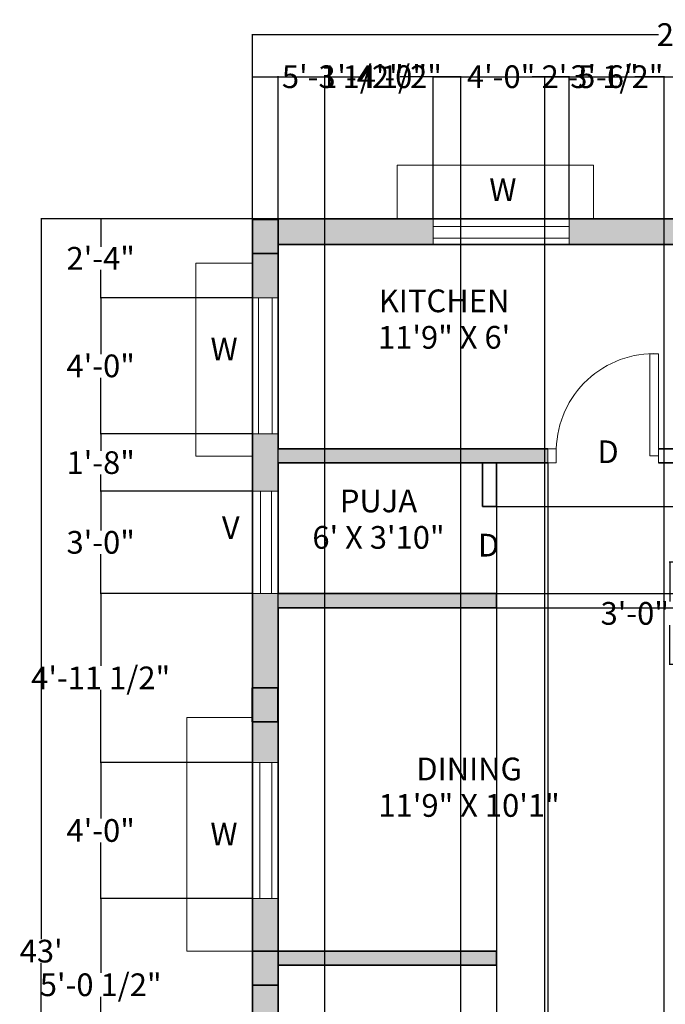
# Model space of a CAD drawing. Units: inches. Extents: x 374 to 1054, y -870 to -188.
# Tile 2 of 3: x 374 to 601, y -535 to -188. Entities that reach past the tile are written whole.
import ezdxf
from ezdxf.enums import TextEntityAlignment as Align

# ---------------------------------------------------------------- set-up
doc = ezdxf.new("R2010")
doc.units = ezdxf.units.IN
doc.header["$MEASUREMENT"] = 0
for name, color, linetype, lineweight, true_color in [('A-ANNO-DIMS', 244, 'Continuous', 18, 0x991b1e), ('A-AREA-IDEN', 116, 'Continuous', 18, 0x136734), ('A-WALL-PATT', 116, 'Continuous', 13, 0x136734)]:
    doc.layers.add(name, color=color, linetype=linetype, lineweight=lineweight, true_color=true_color)
for name, color, linetype, lineweight in [('A-ANNO-TEXT', 7, 'Continuous', 18), ('A-COLS', 1, 'Continuous', 35), ('A-DOOR', 4, 'Continuous', 18), ('A-FLOR-CASE-PATT', 8, 'Continuous', 13), ('A-GLAZ', 4, 'Continuous', 18), ('A-GLAZ-PROJ', 4, 'Continuous', 13), ('A-WALL', 7, 'Continuous', 35)]:
    doc.layers.add(name, color=color, linetype=linetype, lineweight=lineweight)
doc.styles.get("Standard").update_dxf_attribs({"font": 'arial.ttf'})
doc.dimstyles.get("Standard").update_dxf_attribs({"dimtxt": 8, "dimasz": 0.18, "dimexe": 0.18, "dimexo": 0.0625, "dimgap": 0.09, "dimtad": 0, "dimtih": 1, "dimtoh": 1, "dimzin": 0, "dimdsep": 46, "dimlunit": 3, "dimtxsty": 'Standard', "dimcen": 0.09, "dimadec": 0, "dimazin": 0, "dimtfac": 1, "dimtofl": 0, "dimtmove": 0, "dimatfit": 3, "dimfxl": 1, "dimtolj": 1, "dimtzin": 0, "dimarcsym": 0})

# ---------------------------------------------------------------- blocks, each defined once
blk = doc.blocks.new('*D1')
at = {"layer": 'A-ANNO-DIMS', "color": 0, "lineweight": -2, "transparency": 16777216}
for p, q in [((455.9, -257.88), (455.9, -192.83)), ((456.08, -193.01), (598.96, -193.01)), ((755.72, -193.01), (612.85, -193.01)), ((755.9, -257.88), (755.9, -192.83))]:
    blk.add_line(p, q, dxfattribs=at)
at = {"layer": 'A-ANNO-DIMS', "color": 0, "transparency": 16777216}
for points in [[(456.08, -192.98), (456.08, -193.04), (455.9, -193.01)], [(755.72, -192.98), (755.72, -193.04), (755.9, -193.01)]]:
    blk.add_solid(points, dxfattribs=at)
at = {"layer": 'Defpoints', "color": 0, "transparency": 16777216}
for p in [(755.9, -193.01), (455.9, -257.94), (755.9, -257.94)]:
    blk.add_point(p, dxfattribs=at)
at = {"layer": 'A-ANNO-DIMS', "color": 0, "transparency": 16777216, "insert": (605.9, -193.01), "char_height": 8, "attachment_point": 5}
blk.add_mtext("\\A1;25'", dxfattribs=at)
blk = doc.blocks.new('*D2')
at = {"layer": 'A-ANNO-DIMS', "color": 0, "lineweight": -2, "transparency": 16777216}
for p, q in [((455.84, -257.94), (381.2, -257.94)), ((381.38, -258.12), (381.38, -511.76)), ((381.38, -773.76), (381.38, -520.12)), ((455.84, -773.94), (381.2, -773.94))]:
    blk.add_line(p, q, dxfattribs=at)
at = {"layer": 'A-ANNO-DIMS', "color": 0, "transparency": 16777216}
for points in [[(381.35, -258.12), (381.41, -258.12), (381.38, -257.94)], [(381.35, -773.76), (381.41, -773.76), (381.38, -773.94)]]:
    blk.add_solid(points, dxfattribs=at)
at = {"layer": 'Defpoints', "color": 0, "transparency": 16777216}
for p in [(381.38, -257.94), (455.9, -257.94), (455.9, -773.94)]:
    blk.add_point(p, dxfattribs=at)
at = {"layer": 'A-ANNO-DIMS', "color": 0, "transparency": 16777216, "insert": (381.38, -515.94), "char_height": 8, "attachment_point": 5}
blk.add_mtext("\\A1;43'", dxfattribs=at)
blk = doc.blocks.new('COL-12X9')
h = blk.add_hatch(color=256)
h.dxf.hatch_style = 1
h.paths.add_polyline_path([(6, 4.5), (-6, 4.5), (-6, -4.5), (6, -4.5)])
blk.add_lwpolyline([(-6, 4.5), (6, 4.5), (6, -4.5), (-6, -4.5)], close=True)
blk = doc.blocks.new('DOOR-SWING-36')
blk.add_lwpolyline([(0, 0), (-3, 0), (-3, 36), (0, 36)], close=True)
blk.add_arc((-1.5, 1.52), 34.51, 87.5091, 178.3707)
blk = doc.blocks.new('*D9')
at = {"layer": 'A-ANNO-DIMS', "color": 0, "lineweight": -2, "transparency": 16777216}
for p, q in [((608.34, -378.94), (602.76, -378.94)), ((602.94, -379.12), (602.94, -392.76)), ((602.94, -414.76), (602.94, -401.12)), ((608.34, -414.94), (602.76, -414.94))]:
    blk.add_line(p, q, dxfattribs=at)
at = {"layer": 'A-ANNO-DIMS', "color": 0, "transparency": 16777216}
for points in [[(602.91, -379.12), (602.97, -379.12), (602.94, -378.94)], [(602.91, -414.76), (602.97, -414.76), (602.94, -414.94)]]:
    blk.add_solid(points, dxfattribs=at)
at = {"layer": 'Defpoints', "color": 0, "transparency": 16777216}
for p in [(608.4, -378.94), (602.94, -414.94), (608.4, -414.94)]:
    blk.add_point(p, dxfattribs=at)
at = {"layer": 'A-ANNO-DIMS', "color": 0, "transparency": 16777216, "insert": (602.94, -396.94), "char_height": 8, "attachment_point": 5}
blk.add_mtext('\\A1;3\'-0" TYP.', dxfattribs=at)
blk = doc.blocks.new('*D12')
at = {"layer": 'A-ANNO-DIMS', "color": 0, "lineweight": -2, "transparency": 16777216}
for p, q in [((455.9, -257.88), (455.9, -207.66)), ((456.08, -207.84), (467.65, -207.84)), ((519.3, -207.84), (507.74, -207.84)), ((519.48, -257.88), (519.48, -207.66))]:
    blk.add_line(p, q, dxfattribs=at)
at = {"layer": 'A-ANNO-DIMS', "color": 0, "transparency": 16777216}
for points in [[(456.08, -207.81), (456.08, -207.87), (455.9, -207.84)], [(519.3, -207.81), (519.3, -207.87), (519.48, -207.84)]]:
    blk.add_solid(points, dxfattribs=at)
at = {"layer": 'Defpoints', "color": 0, "transparency": 16777216}
for p in [(519.48, -207.84), (455.9, -257.94), (519.48, -257.94)]:
    blk.add_point(p, dxfattribs=at)
at = {"layer": 'A-ANNO-DIMS', "color": 0, "transparency": 16777216, "insert": (487.69, -207.84), "char_height": 8, "attachment_point": 5}
blk.add_mtext('\\A1;5\'-3 1/2"', dxfattribs=at)
blk = doc.blocks.new('*D13')
at = {"layer": 'A-ANNO-DIMS', "color": 0, "lineweight": -2, "transparency": 16777216}
for p, q in [((519.48, -257.88), (519.48, -207.66)), ((519.66, -207.84), (532.6, -207.84)), ((567.3, -207.84), (554.37, -207.84)), ((567.48, -257.88), (567.48, -207.66))]:
    blk.add_line(p, q, dxfattribs=at)
at = {"layer": 'A-ANNO-DIMS', "color": 0, "transparency": 16777216}
for points in [[(519.66, -207.81), (519.66, -207.87), (519.48, -207.84)], [(567.3, -207.81), (567.3, -207.87), (567.48, -207.84)]]:
    blk.add_solid(points, dxfattribs=at)
at = {"layer": 'Defpoints', "color": 0, "transparency": 16777216}
for p in [(567.48, -207.84), (519.48, -257.94), (567.48, -257.94)]:
    blk.add_point(p, dxfattribs=at)
at = {"layer": 'A-ANNO-DIMS', "color": 0, "transparency": 16777216, "insert": (543.48, -207.84), "char_height": 8, "attachment_point": 5}
blk.add_mtext('\\A1;4\'-0"', dxfattribs=at)
blk = doc.blocks.new('*D14')
at = {"layer": 'A-ANNO-DIMS', "color": 0, "lineweight": -2, "transparency": 16777216}
for p, q in [((567.48, -257.88), (567.48, -207.66)), ((567.66, -207.84), (606.87, -207.84)), ((667.53, -207.84), (628.32, -207.84)), ((667.71, -257.88), (667.71, -207.66))]:
    blk.add_line(p, q, dxfattribs=at)
at = {"layer": 'A-ANNO-DIMS', "color": 0, "transparency": 16777216}
for points in [[(567.66, -207.81), (567.66, -207.87), (567.48, -207.84)], [(667.53, -207.81), (667.53, -207.87), (667.71, -207.84)]]:
    blk.add_solid(points, dxfattribs=at)
at = {"layer": 'Defpoints', "color": 0, "transparency": 16777216}
for p in [(667.71, -207.84), (567.48, -257.94), (667.71, -257.94)]:
    blk.add_point(p, dxfattribs=at)
at = {"layer": 'A-ANNO-DIMS', "color": 0, "transparency": 16777216, "insert": (617.6, -207.84), "char_height": 8, "attachment_point": 5}
blk.add_mtext('\\A1;8\'-4"', dxfattribs=at)
blk = doc.blocks.new('*D16')
at = {"layer": 'A-ANNO-DIMS', "color": 0, "lineweight": -2, "transparency": 16777216}
for p, q in [((455.84, -257.94), (402.18, -257.94)), ((402.36, -258.12), (402.36, -267.73)), ((402.36, -285.55), (402.36, -275.94)), ((455.84, -285.73), (402.18, -285.73))]:
    blk.add_line(p, q, dxfattribs=at)
at = {"layer": 'A-ANNO-DIMS', "color": 0, "transparency": 16777216}
for points in [[(402.33, -258.12), (402.39, -258.12), (402.36, -257.94)], [(402.33, -285.55), (402.39, -285.55), (402.36, -285.73)]]:
    blk.add_solid(points, dxfattribs=at)
at = {"layer": 'Defpoints', "color": 0, "transparency": 16777216}
for p in [(455.9, -257.94), (402.36, -285.73), (455.9, -285.73)]:
    blk.add_point(p, dxfattribs=at)
at = {"layer": 'A-ANNO-DIMS', "color": 0, "transparency": 16777216, "insert": (402.36, -271.83), "char_height": 8, "attachment_point": 5}
blk.add_mtext('\\A1;2\'-4"', dxfattribs=at)
blk = doc.blocks.new('*D17')
at = {"layer": 'A-ANNO-DIMS', "color": 0, "lineweight": -2, "transparency": 16777216}
for p, q in [((455.84, -285.73), (402.18, -285.73)), ((402.36, -285.91), (402.36, -305.56)), ((402.36, -333.55), (402.36, -313.9)), ((455.84, -333.73), (402.18, -333.73))]:
    blk.add_line(p, q, dxfattribs=at)
at = {"layer": 'A-ANNO-DIMS', "color": 0, "transparency": 16777216}
for points in [[(402.33, -285.91), (402.39, -285.91), (402.36, -285.73)], [(402.33, -333.55), (402.39, -333.55), (402.36, -333.73)]]:
    blk.add_solid(points, dxfattribs=at)
at = {"layer": 'Defpoints', "color": 0, "transparency": 16777216}
for p in [(455.9, -285.73), (402.36, -333.73), (455.9, -333.73)]:
    blk.add_point(p, dxfattribs=at)
at = {"layer": 'A-ANNO-DIMS', "color": 0, "transparency": 16777216, "insert": (402.36, -309.73), "char_height": 8, "attachment_point": 5}
blk.add_mtext('\\A1;4\'-0"', dxfattribs=at)
blk = doc.blocks.new('*D18')
at = {"layer": 'A-ANNO-DIMS', "color": 0, "lineweight": -2, "transparency": 16777216}
for p, q in [((455.84, -333.73), (402.18, -333.73)), ((402.36, -333.91), (402.36, -339.64)), ((402.36, -353.73), (402.36, -347.99)), ((455.84, -353.91), (402.18, -353.91))]:
    blk.add_line(p, q, dxfattribs=at)
at = {"layer": 'A-ANNO-DIMS', "color": 0, "transparency": 16777216}
for points in [[(402.33, -333.91), (402.39, -333.91), (402.36, -333.73)], [(402.33, -353.73), (402.39, -353.73), (402.36, -353.91)]]:
    blk.add_solid(points, dxfattribs=at)
at = {"layer": 'Defpoints', "color": 0, "transparency": 16777216}
for p in [(455.9, -333.73), (402.36, -353.91), (455.9, -353.91)]:
    blk.add_point(p, dxfattribs=at)
at = {"layer": 'A-ANNO-DIMS', "color": 0, "transparency": 16777216, "insert": (402.36, -343.82), "char_height": 8, "attachment_point": 5}
blk.add_mtext('\\A1;1\'-8"', dxfattribs=at)
blk = doc.blocks.new('*D19')
at = {"layer": 'A-ANNO-DIMS', "color": 0, "lineweight": -2, "transparency": 16777216}
for p, q in [((455.84, -353.91), (402.18, -353.91)), ((402.36, -354.09), (402.36, -367.73)), ((402.36, -389.73), (402.36, -376.09)), ((455.84, -389.91), (402.18, -389.91))]:
    blk.add_line(p, q, dxfattribs=at)
at = {"layer": 'A-ANNO-DIMS', "color": 0, "transparency": 16777216}
for points in [[(402.33, -354.09), (402.39, -354.09), (402.36, -353.91)], [(402.33, -389.73), (402.39, -389.73), (402.36, -389.91)]]:
    blk.add_solid(points, dxfattribs=at)
at = {"layer": 'Defpoints', "color": 0, "transparency": 16777216}
for p in [(455.9, -353.91), (402.36, -389.91), (455.9, -389.91)]:
    blk.add_point(p, dxfattribs=at)
at = {"layer": 'A-ANNO-DIMS', "color": 0, "transparency": 16777216, "insert": (402.36, -371.91), "char_height": 8, "attachment_point": 5}
blk.add_mtext('\\A1;3\'-0"', dxfattribs=at)
blk = doc.blocks.new('*D20')
at = {"layer": 'A-ANNO-DIMS', "color": 0, "lineweight": -2, "transparency": 16777216}
for p, q in [((455.84, -389.91), (402.18, -389.91)), ((402.36, -390.09), (402.36, -415.44)), ((402.36, -449.25), (402.36, -423.9)), ((455.84, -449.43), (402.18, -449.43))]:
    blk.add_line(p, q, dxfattribs=at)
at = {"layer": 'A-ANNO-DIMS', "color": 0, "transparency": 16777216}
for points in [[(402.33, -390.09), (402.39, -390.09), (402.36, -389.91)], [(402.33, -449.25), (402.39, -449.25), (402.36, -449.43)]]:
    blk.add_solid(points, dxfattribs=at)
at = {"layer": 'Defpoints', "color": 0, "transparency": 16777216}
for p in [(455.9, -389.91), (402.36, -449.43), (455.9, -449.43)]:
    blk.add_point(p, dxfattribs=at)
at = {"layer": 'A-ANNO-DIMS', "color": 0, "transparency": 16777216, "insert": (402.36, -419.67), "char_height": 8, "attachment_point": 5}
blk.add_mtext('\\A1;4\'-11 1/2"', dxfattribs=at)
blk = doc.blocks.new('*D21')
at = {"layer": 'A-ANNO-DIMS', "color": 0, "lineweight": -2, "transparency": 16777216}
for p, q in [((455.84, -449.43), (402.18, -449.43)), ((402.36, -449.61), (402.36, -469.26)), ((402.36, -497.25), (402.36, -477.61)), ((455.84, -497.43), (402.18, -497.43))]:
    blk.add_line(p, q, dxfattribs=at)
at = {"layer": 'A-ANNO-DIMS', "color": 0, "transparency": 16777216}
for points in [[(402.33, -449.61), (402.39, -449.61), (402.36, -449.43)], [(402.33, -497.25), (402.39, -497.25), (402.36, -497.43)]]:
    blk.add_solid(points, dxfattribs=at)
at = {"layer": 'Defpoints', "color": 0, "transparency": 16777216}
for p in [(455.9, -449.43), (402.36, -497.43), (455.9, -497.43)]:
    blk.add_point(p, dxfattribs=at)
at = {"layer": 'A-ANNO-DIMS', "color": 0, "transparency": 16777216, "insert": (402.36, -473.43), "char_height": 8, "attachment_point": 5}
blk.add_mtext('\\A1;4\'-0"', dxfattribs=at)
blk = doc.blocks.new('*D22')
at = {"layer": 'A-ANNO-DIMS', "color": 0, "lineweight": -2, "transparency": 16777216}
for p, q in [((455.84, -497.43), (402.18, -497.43)), ((402.36, -497.61), (402.36, -523.56)), ((402.36, -557.96), (402.36, -532.01)), ((455.84, -558.14), (402.18, -558.14))]:
    blk.add_line(p, q, dxfattribs=at)
at = {"layer": 'A-ANNO-DIMS', "color": 0, "transparency": 16777216}
for points in [[(402.33, -497.61), (402.39, -497.61), (402.36, -497.43)], [(402.33, -557.96), (402.39, -557.96), (402.36, -558.14)]]:
    blk.add_solid(points, dxfattribs=at)
at = {"layer": 'Defpoints', "color": 0, "transparency": 16777216}
for p in [(455.9, -497.43), (402.36, -558.14), (455.9, -558.14)]:
    blk.add_point(p, dxfattribs=at)
at = {"layer": 'A-ANNO-DIMS', "color": 0, "transparency": 16777216, "insert": (402.36, -527.79), "char_height": 8, "attachment_point": 5}
blk.add_mtext('\\A1;5\'-0 1/2"', dxfattribs=at)
blk = doc.blocks.new('*D25')
at = {"layer": 'A-ANNO-DIMS', "color": 0, "lineweight": -2, "transparency": 16777216}
for p, q in [((541.93, -389.94), (810.73, -389.94)), ((810.55, -390.12), (810.55, -394.76)), ((541.92, -394.94), (810.73, -394.94)), ((810.55, -395.12), (810.37, -395.12)), ((810.55, -394.94), (810.55, -395.12))]:
    blk.add_line(p, q, dxfattribs=at)
at = {"layer": 'A-ANNO-DIMS', "color": 0, "transparency": 16777216}
for points in [[(810.52, -390.12), (810.58, -390.12), (810.55, -389.94)], [(810.52, -394.76), (810.58, -394.76), (810.55, -394.94)]]:
    blk.add_solid(points, dxfattribs=at)
at = {"layer": 'Defpoints', "color": 0, "transparency": 16777216}
for p in [(541.86, -389.94), (541.86, -394.94), (810.55, -394.94)]:
    blk.add_point(p, dxfattribs=at)
at = {"layer": 'A-ANNO-DIMS', "color": 0, "transparency": 16777216, "insert": (799.65, -395.12), "char_height": 8, "attachment_point": 5}
blk.add_mtext('\\A1;0\'-5"', dxfattribs=at)
blk = doc.blocks.new('*D39')
at = {"layer": 'A-ANNO-DIMS', "color": 0, "lineweight": -2, "transparency": 16777216}
for p, q in [((464.9, -680.88), (464.9, -207.66)), ((465.08, -207.84), (481.13, -207.84)), ((481.31, -680.88), (481.31, -207.66)), ((481.31, -207.84), (481.49, -207.84))]:
    blk.add_line(p, q, dxfattribs=at)
at = {"layer": 'A-ANNO-DIMS', "color": 0, "transparency": 16777216}
for points in [[(465.08, -207.81), (465.08, -207.87), (464.9, -207.84)], [(481.13, -207.81), (481.13, -207.87), (481.31, -207.84)]]:
    blk.add_solid(points, dxfattribs=at)
at = {"layer": 'Defpoints', "color": 0, "transparency": 16777216}
for p in [(481.31, -207.84), (464.9, -680.94), (481.31, -680.94)]:
    blk.add_point(p, dxfattribs=at)
at = {"layer": 'A-ANNO-DIMS', "color": 0, "transparency": 16777216, "insert": (501.16, -207.84), "char_height": 8, "attachment_point": 5}
blk.add_mtext('\\A1;1\'-4 1/2"', dxfattribs=at)
blk = doc.blocks.new('*D40')
at = {"layer": 'A-ANNO-DIMS', "color": 0, "lineweight": -2, "transparency": 16777216}
for p, q in [((481.31, -680.88), (481.31, -207.66)), ((481.49, -207.84), (494.43, -207.84)), ((529.13, -207.84), (516.2, -207.84)), ((529.31, -680.88), (529.31, -207.66))]:
    blk.add_line(p, q, dxfattribs=at)
at = {"layer": 'A-ANNO-DIMS', "color": 0, "transparency": 16777216}
for points in [[(481.49, -207.81), (481.49, -207.87), (481.31, -207.84)], [(529.13, -207.81), (529.13, -207.87), (529.31, -207.84)]]:
    blk.add_solid(points, dxfattribs=at)
at = {"layer": 'Defpoints', "color": 0, "transparency": 16777216}
for p in [(529.31, -207.84), (481.31, -680.94), (529.31, -680.94)]:
    blk.add_point(p, dxfattribs=at)
at = {"layer": 'A-ANNO-DIMS', "color": 0, "transparency": 16777216, "insert": (505.31, -207.84), "char_height": 8, "attachment_point": 5}
blk.add_mtext('\\A1;4\'-0"', dxfattribs=at)
blk = doc.blocks.new('*D41')
at = {"layer": 'A-ANNO-DIMS', "color": 0, "lineweight": -2, "transparency": 16777216}
for p, q in [((529.31, -680.88), (529.31, -207.66)), ((529.49, -207.84), (558.72, -207.84)), ((558.9, -680.88), (558.9, -207.66)), ((558.9, -207.84), (559.08, -207.84))]:
    blk.add_line(p, q, dxfattribs=at)
at = {"layer": 'A-ANNO-DIMS', "color": 0, "transparency": 16777216}
for points in [[(529.49, -207.81), (529.49, -207.87), (529.31, -207.84)], [(558.72, -207.81), (558.72, -207.87), (558.9, -207.84)]]:
    blk.add_solid(points, dxfattribs=at)
at = {"layer": 'Defpoints', "color": 0, "transparency": 16777216}
for p in [(558.9, -207.84), (529.31, -680.94), (558.9, -680.94)]:
    blk.add_point(p, dxfattribs=at)
at = {"layer": 'A-ANNO-DIMS', "color": 0, "transparency": 16777216, "insert": (579.2, -207.84), "char_height": 8, "attachment_point": 5}
blk.add_mtext('\\A1;2\'-5 1/2"', dxfattribs=at)
blk = doc.blocks.new('*D42')
at = {"layer": 'A-ANNO-DIMS', "color": 0, "lineweight": -2, "transparency": 16777216}
for p, q in [((558.9, -680.88), (558.9, -207.66)), ((559.08, -207.84), (569.18, -207.84)), ((600.72, -207.84), (590.63, -207.84)), ((600.9, -680.88), (600.9, -207.66))]:
    blk.add_line(p, q, dxfattribs=at)
at = {"layer": 'A-ANNO-DIMS', "color": 0, "transparency": 16777216}
for points in [[(559.08, -207.81), (559.08, -207.87), (558.9, -207.84)], [(600.72, -207.81), (600.72, -207.87), (600.9, -207.84)]]:
    blk.add_solid(points, dxfattribs=at)
at = {"layer": 'Defpoints', "color": 0, "transparency": 16777216}
for p in [(600.9, -207.84), (558.9, -680.94), (600.9, -680.94)]:
    blk.add_point(p, dxfattribs=at)
at = {"layer": 'A-ANNO-DIMS', "color": 0, "transparency": 16777216, "insert": (579.9, -207.84), "char_height": 8, "attachment_point": 5}
blk.add_mtext('\\A1;3\'-6"', dxfattribs=at)
blk = doc.blocks.new('*D45')
at = {"layer": 'A-ANNO-DIMS', "color": 0, "lineweight": -2, "transparency": 16777216}
for p, q in [((541.9, -344), (541.9, -822.55)), ((559.9, -344), (559.9, -822.55)), ((542.08, -822.37), (559.72, -822.37)), ((559.9, -822.37), (560.08, -822.37))]:
    blk.add_line(p, q, dxfattribs=at)
at = {"layer": 'A-ANNO-DIMS', "color": 0, "transparency": 16777216}
for points in [[(542.08, -822.34), (542.08, -822.4), (541.9, -822.37)], [(559.72, -822.34), (559.72, -822.4), (559.9, -822.37)]]:
    blk.add_solid(points, dxfattribs=at)
at = {"layer": 'Defpoints', "color": 0, "transparency": 16777216}
for p in [(541.9, -343.94), (559.9, -343.94), (559.9, -822.37)]:
    blk.add_point(p, dxfattribs=at)
at = {"layer": 'A-ANNO-DIMS', "color": 0, "transparency": 16777216, "insert": (570.43, -822.37), "char_height": 8, "attachment_point": 5}
blk.add_mtext('\\A1;1\'-6"', dxfattribs=at)
blk = doc.blocks.new('*D46')
at = {"layer": 'A-ANNO-DIMS', "color": 0, "lineweight": -2, "transparency": 16777216}
for p, q in [((541.95, -359.22), (810.73, -359.22)), ((810.55, -359.4), (810.55, -370.35)), ((810.55, -389.76), (810.55, -378.81)), ((541.93, -389.94), (810.73, -389.94))]:
    blk.add_line(p, q, dxfattribs=at)
at = {"layer": 'A-ANNO-DIMS', "color": 0, "transparency": 16777216}
for points in [[(810.52, -359.4), (810.58, -359.4), (810.55, -359.22)], [(810.52, -389.76), (810.58, -389.76), (810.55, -389.94)]]:
    blk.add_solid(points, dxfattribs=at)
at = {"layer": 'Defpoints', "color": 0, "transparency": 16777216}
for p in [(541.89, -359.22), (541.86, -389.94), (810.55, -389.94)]:
    blk.add_point(p, dxfattribs=at)
at = {"layer": 'A-ANNO-DIMS', "color": 0, "transparency": 16777216, "insert": (810.55, -374.58), "char_height": 8, "attachment_point": 5}
blk.add_mtext('\\A1;2\'-6 1/2"', dxfattribs=at)

msp = doc.modelspace()

# ---------------------------------------------------------------- hatches: boundary and pattern name
at = {"layer": 'A-FLOR-CASE-PATT'}
h = msp.add_hatch(dxfattribs=at)
h.set_pattern_fill('AR-HBONE', color=256)
h.paths.add_polyline_path([(638.563, -266.938), (610.905, -266.938), (610.905, -343.938), (610.905, -361.438), (638.563, -361.438)])
h.paths.add_polyline_path([(620.136, -288.822), (620.136, -356.301), (632.553, -356.301), (632.553, -288.822)], flags=24)
h.paths.add_polyline_path([(727.152, -700.465), (727.152, -761.497), (739.414, -761.497), (739.414, -700.465)], flags=9)
h.paths.add_polyline_path([(497.837, -702.053), (512.386, -702.053), (512.386, -690.053), (497.837, -690.053)], flags=9)
h.paths.add_polyline_path([(494.709, -751.886), (551.702, -751.886), (551.702, -739.837), (494.709, -739.837)], flags=9)
h.paths.add_polyline_path([(490.155, -739.027), (556.256, -739.027), (556.256, -727.027), (490.155, -727.027)], flags=9)
h.paths.add_polyline_path([(488.741, -637.8), (555.988, -637.8), (555.988, -625.538), (488.741, -625.538)], flags=9)
h.paths.add_polyline_path([(501.975, -624.968), (542.755, -624.968), (542.755, -612.559), (501.975, -612.559)], flags=9)
h.paths.add_polyline_path([(498.568, -470.79), (565.812, -470.79), (565.812, -458.536), (498.568, -458.536)], flags=9)
h.paths.add_polyline_path([(510.563, -457.965), (553.816, -457.965), (553.816, -445.555), (510.563, -445.555)], flags=9)
h.paths.add_polyline_path([(474.841, -376.354), (525.689, -376.354), (525.689, -364.092), (474.841, -364.092)], flags=9)
h.paths.add_polyline_path([(483.939, -363.488), (516.591, -363.488), (516.591, -351.283), (483.939, -351.283)], flags=9)
h.paths.add_polyline_path([(652.121, -604.662), (719.368, -604.662), (719.368, -592.4), (652.121, -592.4)], flags=9)
h.paths.add_polyline_path([(650.141, -591.831), (721.347, -591.831), (721.347, -579.414), (650.141, -579.414)], flags=9)
h.paths.add_polyline_path([(613.577, -603.955), (613.577, -672.673), (625.995, -672.673), (625.995, -603.955)], flags=9)
h.paths.add_polyline_path([(704.619, -508.492), (742.954, -508.492), (742.954, -496.492), (704.619, -496.492)], flags=9)
h.paths.add_polyline_path([(706.883, -495.641), (740.69, -495.641), (740.69, -483.641), (706.883, -483.641)], flags=9)
h.paths.add_polyline_path([(695.312, -483.057), (752.261, -483.057), (752.261, -470.566), (695.312, -470.566)], flags=9)
h.paths.add_polyline_path([(699.358, -470.143), (748.215, -470.143), (748.215, -457.734), (699.358, -457.734)], flags=9)
h.paths.add_polyline_path([(623.681, -465.885), (684.71, -465.885), (684.71, -453.631), (623.681, -453.631)], flags=9)
h.paths.add_polyline_path([(611.019, -455.848), (697.775, -455.848), (697.775, -443.357), (611.019, -443.357)], flags=9)
h.paths.add_polyline_path([(625.622, -442.934), (683.172, -442.934), (683.172, -430.525), (625.622, -430.525)], flags=9)
at = {"layer": 'A-WALL-PATT'}
h = msp.add_hatch(color=256, dxfattribs=at)
h.dxf.hatch_style = 1
h.paths.add_polyline_path([(667.71, -257.938), (614.905, -257.938), (614.905, -266.938), (667.71, -266.938)])
h.paths.add_polyline_path([(746.905, -257.938), (715.71, -257.938), (715.71, -266.938), (746.905, -266.938)])
h.paths.add_polyline_path([(755.905, -270.034), (746.905, -270.034), (746.905, -327.137), (755.905, -327.137)])
h.paths.add_polyline_path([(755.905, -375.137), (746.905, -375.137), (746.905, -422.975), (755.905, -422.975)])
h.paths.add_polyline_path([(605.905, -257.938), (567.481, -257.938), (567.481, -266.938), (605.905, -266.938)])
h.paths.add_polyline_path([(519.481, -257.938), (464.905, -257.938), (464.905, -266.938), (519.481, -266.938)])
h.paths.add_polyline_path([(464.905, -270.108), (455.905, -270.108), (455.905, -285.73), (464.905, -285.73)])
h.paths.add_polyline_path([(464.905, -343.938), (559.905, -343.938), (559.905, -338.938), (464.905, -338.938), (464.905, -333.73), (455.905, -333.73), (455.905, -353.908), (464.905, -353.908)])
h.paths.add_polyline_path([(464.905, -394.938), (541.859, -394.938), (541.863, -389.942), (536.905, -389.938), (464.905, -389.938), (455.905, -389.908), (455.905, -423.118), (464.905, -423.118)])
h.paths.add_polyline_path([(464.905, -435.118), (455.905, -435.118), (455.905, -449.434), (464.905, -449.434)])
h.paths.add_polyline_path([(464.905, -497.434), (455.905, -497.434), (455.905, -515.926), (464.905, -515.926)])
h.paths.add_polyline_path([(464.905, -527.926), (455.905, -527.926), (455.905, -558.14), (464.905, -558.14)])
h.paths.add_polyline_path([(755.905, -489.995), (746.905, -489.995), (746.905, -515.947), (755.905, -515.947)])
h.paths.add_polyline_path([(755.905, -434.975), (746.905, -434.975), (746.905, -453.995), (755.905, -453.995)])
h.paths.add_polyline_path([(746.905, -422.938), (738.905, -422.938), (738.905, -427.938), (746.905, -427.938)])
h.paths.add_polyline_path([(614.905, -423.118), (614.905, -435.118), (605.905, -435.118), (605.905, -423.118), (605.905, -417.938), (610.905, -417.938), (610.905, -423.118)])
h.paths.add_polyline_path([(610.905, -435.118), (605.905, -435.118), (605.905, -469.938), (610.905, -469.938)])
h.paths.add_polyline_path([(541.859, -515.938), (464.905, -515.938), (464.905, -520.938), (541.859, -520.938)])
h.paths.add_polyline_path([(755.905, -527.947), (746.905, -527.947), (746.905, -581.613), (755.905, -581.613)])
h.paths.add_polyline_path([(755.905, -629.613), (746.905, -629.613), (746.905, -677.938), (755.905, -677.938)])
h.paths.add_polyline_path([(755.905, -689.938), (746.905, -689.938), (746.905, -764.938), (755.905, -764.938)])
h.paths.add_polyline_path([(746.905, -680.938), (683.247, -680.938), (683.247, -689.938), (746.905, -689.938)])
h.paths.add_polyline_path([(743.737, -764.938), (701.105, -764.938), (701.105, -773.938), (743.737, -773.938)])
h.paths.add_polyline_path([(653.105, -764.938), (617.905, -764.938), (617.905, -773.938), (653.105, -773.938)])
h.paths.add_polyline_path([(635.247, -680.938), (614.944, -680.938), (614.944, -689.938), (635.247, -689.938)])
h.paths.add_polyline_path([(610.905, -567.938), (605.905, -567.938), (605.905, -677.938), (610.905, -677.938)])
h.paths.add_polyline_path([(558.905, -680.938), (529.314, -680.938), (529.314, -687.485), (529.314, -689.938), (558.905, -689.938)])
h.paths.add_polyline_path([(481.314, -680.938), (464.905, -680.938), (464.905, -689.938), (481.314, -689.938)])
h.paths.add_polyline_path([(464.905, -606.14), (455.905, -606.14), (455.905, -677.938), (464.905, -677.938)])
h.paths.add_polyline_path([(601.753, -550.416), (613.824, -550.416), (613.824, -538.416), (601.753, -538.416)], flags=9)
h.paths.add_polyline_path([(604.254, -492.526), (616.325, -492.526), (616.325, -480.526), (604.254, -480.526)], flags=9)
h.paths.add_polyline_path([(604.661, -400.451), (616.732, -400.451), (616.732, -388.451), (604.661, -388.451)], flags=9)
h.paths.add_polyline_path([(533.025, -378.901), (545.096, -378.901), (545.096, -366.901), (533.025, -366.901)], flags=9)
h.paths.add_polyline_path([(575.128, -346.003), (587.199, -346.003), (587.199, -334.003), (575.128, -334.003)], flags=9)
h.paths.add_polyline_path([(488.741, -637.8), (555.988, -637.8), (555.988, -625.538), (488.741, -625.538)], flags=9)
h.paths.add_polyline_path([(501.975, -624.968), (542.755, -624.968), (542.755, -612.559), (501.975, -612.559)], flags=9)
h.paths.add_polyline_path([(498.568, -470.79), (565.812, -470.79), (565.812, -458.536), (498.568, -458.536)], flags=9)
h.paths.add_polyline_path([(510.563, -457.965), (553.816, -457.965), (553.816, -445.555), (510.563, -445.555)], flags=9)
h.paths.add_polyline_path([(474.841, -376.354), (525.689, -376.354), (525.689, -364.092), (474.841, -364.092)], flags=9)
h.paths.add_polyline_path([(483.939, -363.488), (516.591, -363.488), (516.591, -351.283), (483.939, -351.283)], flags=9)
h.paths.add_polyline_path([(652.121, -604.662), (719.368, -604.662), (719.368, -592.4), (652.121, -592.4)], flags=9)
h.paths.add_polyline_path([(650.141, -591.831), (721.347, -591.831), (721.347, -579.414), (650.141, -579.414)], flags=9)
h.paths.add_polyline_path([(715.698, -427.661), (727.769, -427.661), (727.769, -415.661), (715.698, -415.661)], flags=9)
h.paths.add_polyline_path([(573.757, -690.34), (585.828, -690.34), (585.828, -678.34), (573.757, -678.34)], flags=9)
h.paths.add_polyline_path([(727.152, -700.465), (727.152, -761.497), (739.414, -761.497), (739.414, -700.465)], flags=9)
h.paths.add_polyline_path([(497.837, -702.053), (512.386, -702.053), (512.386, -690.053), (497.837, -690.053)], flags=9)
h.paths.add_polyline_path([(494.709, -751.886), (551.702, -751.886), (551.702, -739.837), (494.709, -739.837)], flags=9)
h.paths.add_polyline_path([(490.155, -739.027), (556.256, -739.027), (556.256, -727.027), (490.155, -727.027)], flags=9)
h.paths.add_polyline_path([(613.577, -603.955), (613.577, -672.673), (625.995, -672.673), (625.995, -603.955)], flags=9)
h.paths.add_polyline_path([(695.312, -483.057), (752.261, -483.057), (752.261, -470.566), (695.312, -470.566)], flags=9)
h.paths.add_polyline_path([(611.019, -455.848), (697.775, -455.848), (697.775, -443.357), (611.019, -443.357)], flags=9)
h.paths.add_polyline_path([(663.069, -377.631), (720.133, -377.631), (720.133, -365.369), (663.069, -365.369)], flags=9)
h.paths.add_polyline_path([(657.829, -364.537), (729.035, -364.537), (729.035, -352.12), (657.829, -352.12)], flags=9)
h.paths.add_polyline_path([(620.136, -288.822), (620.136, -356.301), (632.553, -356.301), (632.553, -288.822)], flags=9)
h.paths.add_polyline_path([(497.968, -305.851), (548.814, -305.851), (548.814, -293.597), (497.968, -293.597)], flags=9)
h.paths.add_polyline_path([(496.797, -293.026), (549.986, -293.026), (549.986, -280.617), (496.797, -280.617)], flags=9)
h = msp.add_hatch(color=256, dxfattribs=at)
h.dxf.hatch_style = 1
h.paths.add_polyline_path([(705.905, -425.438), (705.905, -422.938), (610.905, -422.938), (610.905, -417.938), (605.905, -417.938), (605.905, -469.938), (610.905, -469.938), (610.905, -435.118), (610.905, -427.938), (693.905, -427.938), (698.905, -427.938), (705.905, -427.938)])
h.paths.add_polyline_path([(715.698, -427.661), (727.769, -427.661), (727.769, -415.661), (715.698, -415.661)], flags=9)
h.paths.add_polyline_path([(573.757, -690.34), (585.828, -690.34), (585.828, -678.34), (573.757, -678.34)], flags=9)
h.paths.add_polyline_path([(601.753, -550.416), (613.824, -550.416), (613.824, -538.416), (601.753, -538.416)], flags=9)
h.paths.add_polyline_path([(604.254, -492.526), (616.325, -492.526), (616.325, -480.526), (604.254, -480.526)], flags=9)
h.paths.add_polyline_path([(604.661, -400.451), (616.732, -400.451), (616.732, -388.451), (604.661, -388.451)], flags=9)
h.paths.add_polyline_path([(533.025, -378.901), (545.096, -378.901), (545.096, -366.901), (533.025, -366.901)], flags=9)
h.paths.add_polyline_path([(575.128, -346.003), (587.199, -346.003), (587.199, -334.003), (575.128, -334.003)], flags=9)
h.paths.add_polyline_path([(727.152, -700.465), (727.152, -761.497), (739.414, -761.497), (739.414, -700.465)], flags=9)
h.paths.add_polyline_path([(497.837, -702.053), (512.386, -702.053), (512.386, -690.053), (497.837, -690.053)], flags=9)
h.paths.add_polyline_path([(494.709, -751.886), (551.702, -751.886), (551.702, -739.837), (494.709, -739.837)], flags=9)
h.paths.add_polyline_path([(490.155, -739.027), (556.256, -739.027), (556.256, -727.027), (490.155, -727.027)], flags=9)
h.paths.add_polyline_path([(488.741, -637.8), (555.988, -637.8), (555.988, -625.538), (488.741, -625.538)], flags=9)
h.paths.add_polyline_path([(501.975, -624.968), (542.755, -624.968), (542.755, -612.559), (501.975, -612.559)], flags=9)
h.paths.add_polyline_path([(498.568, -470.79), (565.812, -470.79), (565.812, -458.536), (498.568, -458.536)], flags=9)
h.paths.add_polyline_path([(510.563, -457.965), (553.816, -457.965), (553.816, -445.555), (510.563, -445.555)], flags=9)
h.paths.add_polyline_path([(474.841, -376.354), (525.689, -376.354), (525.689, -364.092), (474.841, -364.092)], flags=9)
h.paths.add_polyline_path([(483.939, -363.488), (516.591, -363.488), (516.591, -351.283), (483.939, -351.283)], flags=9)
h.paths.add_polyline_path([(652.121, -604.662), (719.368, -604.662), (719.368, -592.4), (652.121, -592.4)], flags=9)
h.paths.add_polyline_path([(650.141, -591.831), (721.347, -591.831), (721.347, -579.414), (650.141, -579.414)], flags=9)
h.paths.add_polyline_path([(613.577, -603.955), (613.577, -672.673), (625.995, -672.673), (625.995, -603.955)], flags=9)
h.paths.add_polyline_path([(704.619, -508.492), (742.954, -508.492), (742.954, -496.492), (704.619, -496.492)], flags=9)
h.paths.add_polyline_path([(706.883, -495.641), (740.69, -495.641), (740.69, -483.641), (706.883, -483.641)], flags=9)
h.paths.add_polyline_path([(695.312, -483.057), (752.261, -483.057), (752.261, -470.566), (695.312, -470.566)], flags=9)
h.paths.add_polyline_path([(699.358, -470.143), (748.215, -470.143), (748.215, -457.734), (699.358, -457.734)], flags=9)
h.paths.add_polyline_path([(623.681, -465.885), (684.71, -465.885), (684.71, -453.631), (623.681, -453.631)], flags=25)
h.paths.add_polyline_path([(611.019, -455.848), (697.775, -455.848), (697.775, -443.357), (611.019, -443.357)], flags=25)
h.paths.add_polyline_path([(625.622, -442.934), (683.172, -442.934), (683.172, -430.525), (625.622, -430.525)], flags=25)
h.paths.add_polyline_path([(663.069, -377.631), (720.133, -377.631), (720.133, -365.369), (663.069, -365.369)], flags=9)
h.paths.add_polyline_path([(657.829, -364.537), (729.035, -364.537), (729.035, -352.12), (657.829, -352.12)], flags=9)
h.paths.add_polyline_path([(620.136, -288.822), (620.136, -356.301), (632.553, -356.301), (632.553, -288.822)], flags=9)
h.paths.add_polyline_path([(497.968, -305.851), (548.814, -305.851), (548.814, -293.597), (497.968, -293.597)], flags=9)
h.paths.add_polyline_path([(496.797, -293.026), (549.986, -293.026), (549.986, -280.617), (496.797, -280.617)], flags=9)

# ---------------------------------------------------------------- linework, layer by layer
at = {"layer": 'A-DOOR'}
for p, q in [((559.905, -338.938), (559.905, -343.938)), ((559.905, -338.938), (562.905, -338.938)), ((562.905, -338.938), (562.905, -343.938)), ((598.905, -338.938), (598.905, -343.938)), ((562.905, -343.938), (559.905, -343.938))]:
    msp.add_line(p, q, dxfattribs=at)
at = {"layer": 'A-GLAZ'}
for p, q in [((519.481, -257.938), (519.481, -266.938)), ((567.481, -257.938), (567.481, -266.938)), ((519.481, -260.598), (567.481, -260.598)), ((567.481, -264.741), (519.481, -264.741)), ((464.905, -285.73), (455.905, -285.73)), ((457.915, -285.73), (457.915, -333.73)), ((462.82, -285.73), (462.82, -333.73)), ((464.905, -333.73), (455.905, -333.73)), ((464.905, -353.908), (455.905, -353.908)), ((458.687, -389.908), (458.687, -353.908)), ((462.596, -353.908), (462.596, -389.908)), ((464.905, -389.908), (455.905, -389.908)), ((464.905, -449.434), (455.905, -449.434)), ((458.492, -449.434), (458.492, -497.434)), ((462.645, -497.434), (462.645, -449.434)), ((464.905, -497.434), (455.905, -497.434))]:
    msp.add_line(p, q, dxfattribs=at)
at = {"layer": 'A-GLAZ-PROJ'}
for p, q in [((506.871, -257.938), (506.871, -238.981)), ((506.871, -238.981), (575.995, -238.981)), ((575.995, -238.981), (575.995, -257.938)), ((435.835, -341.581), (435.835, -273.525)), ((435.835, -273.525), (455.905, -273.525)), ((455.905, -341.581), (435.835, -341.581)), ((432.751, -515.938), (432.751, -433.646)), ((432.751, -433.646), (455.905, -433.646)), ((455.905, -515.938), (432.751, -515.938))]:
    msp.add_line(p, q, dxfattribs=at)
at = {"layer": 'A-WALL'}
for p, q in [((464.905, -266.938), (605.905, -266.938)), ((464.905, -338.938), (464.905, -266.938)), ((464.905, -338.938), (559.905, -338.938)), ((598.905, -338.938), (605.905, -338.938)), ((464.905, -343.938), (559.905, -343.938)), ((464.905, -389.938), (464.905, -343.938)), ((536.905, -359.22), (536.905, -343.938)), ((541.891, -359.22), (541.905, -343.938)), ((598.905, -343.938), (605.905, -343.938)), ((541.891, -359.22), (536.905, -359.22)), ((464.905, -389.938), (536.905, -389.938)), ((536.905, -389.938), (541.863, -389.942)), ((541.859, -394.938), (541.863, -389.942)), ((464.905, -394.938), (541.859, -394.938)), ((464.905, -680.938), (464.905, -394.938)), ((464.905, -515.938), (541.859, -515.938)), ((541.859, -520.938), (541.859, -515.938)), ((464.905, -520.938), (541.859, -520.938))]:
    msp.add_line(p, q, dxfattribs=at)
msp.add_lwpolyline([(455.905, -257.938), (755.905, -257.938), (755.905, -773.938), (455.905, -773.938)], close=True, dxfattribs=at)

# ---------------------------------------------------------------- block references
at = {"layer": 'A-COLS'}
for p, rotation in [((460.405, -264.108), 269.9999999999991), ((460.247, -429.118), 269.9999999999994), ((460.405, -521.926), 269.9999999999991)]:
    msp.add_blockref('COL-12X9', p, dxfattribs=dict(at, rotation=rotation))
at = {"layer": 'A-DOOR'}
msp.add_blockref('DOOR-SWING-36', (598.905, -341.438), dxfattribs=at)

# ---------------------------------------------------------------- texts
at = {"layer": 'A-ANNO-TEXT'}
for s, p in [('W', (544.095, -251.69)), ('W', (445.848, -307.807)), ('D', (581.164, -344.003)), ('V', (448.192, -370.704)), ('D', (539.06, -376.901)), ('W', (445.793, -478.718))]:
    msp.add_text(s, height=8, dxfattribs=at).set_placement(p, align=Align.CENTER)
at = {"layer": 'A-AREA-IDEN'}
for s, p in [('KITCHEN', (523.391, -290.821)), ('11\'9" X 6\'', (523.391, -303.672)), ('PUJA', (500.265, -361.317)), ('6\' X 3\'10"', (500.265, -374.169)), ('DINING', (532.19, -455.76)), ('11\'9" X 10\'1"', (532.19, -468.611))]:
    msp.add_text(s, height=8, dxfattribs=at).set_placement(p, align=Align.CENTER)

# ---------------------------------------------------------------- dimensions: what is measured, and where the dimension line sits
at = {"layer": 'A-ANNO-DIMS'}
for base, p1, p2, override, picture, middle in [((755.905, -193.005), (455.905, -257.938), (755.905, -257.938), {"dimclrd": 0, "dimclre": 0, "dimclrt": 0}, '*D1', (605.905, -193.005)), ((519.481, -207.841), (455.905, -257.938), (519.481, -257.938), {"dimdec": 1, "dimlfac": 1, "dimrnd": 0, "dimzin": 1, "dimdsep": 46, "dimlunit": 4, "dimfrac": 2}, '*D12', (487.693, -207.841)), ((481.314, -207.841), (464.905, -680.938), (481.314, -680.938), {"dimdec": 1, "dimlfac": 1, "dimrnd": 0, "dimzin": 1, "dimdsep": 46, "dimlunit": 4, "dimfrac": 2}, '*D39', (501.161, -207.841)), ((558.905, -207.841), (529.314, -680.938), (558.905, -680.938), {"dimdec": 1, "dimlfac": 1, "dimrnd": 0, "dimzin": 1, "dimdsep": 46, "dimlunit": 4, "dimfrac": 2}, '*D41', (579.197, -207.841)), ((529.314, -207.841), (481.314, -680.938), (529.314, -680.938), {"dimdec": 1, "dimlfac": 1, "dimrnd": 0, "dimzin": 1, "dimdsep": 46, "dimlunit": 4, "dimfrac": 2}, '*D40', (505.314, -207.841)), ((567.481, -207.841), (519.481, -257.938), (567.481, -257.938), {"dimdec": 1, "dimlfac": 1, "dimrnd": 0, "dimzin": 1, "dimdsep": 46, "dimlunit": 4, "dimfrac": 2}, '*D13', (543.481, -207.841)), ((600.905, -207.841), (558.905, -680.938), (600.905, -680.938), {"dimdec": 1, "dimlfac": 1, "dimrnd": 0, "dimzin": 1, "dimdsep": 46, "dimlunit": 4, "dimfrac": 2}, '*D42', (579.905, -207.841)), ((667.71, -207.841), (567.481, -257.938), (667.71, -257.938), {"dimdec": 1, "dimlfac": 1, "dimrnd": 0, "dimzin": 1, "dimdsep": 46, "dimlunit": 4, "dimfrac": 2}, '*D14', (617.596, -207.841)), ((559.905, -822.366), (541.905, -343.938), (559.905, -343.938), {"dimdec": 1, "dimlfac": 1, "dimrnd": 0, "dimzin": 1, "dimdsep": 46, "dimlunit": 4, "dimfrac": 2}, '*D45', (570.431, -822.366))]:
    dim = msp.add_linear_dim(base=base, p1=p1, p2=p2, dimstyle='Standard', override=override, dxfattribs=at)
    dim.commit()
    dim.dimension.update_dxf_attribs({"geometry": picture, "text_midpoint": middle})
for base, p1, p2, override, picture, middle in [((381.378, -257.938), (455.905, -773.938), (455.905, -257.938), {"dimclrd": 0, "dimclre": 0, "dimclrt": 0}, '*D2', (381.378, -515.938)), ((402.361, -285.73), (455.905, -257.938), (455.905, -285.73), {"dimdec": 1, "dimlfac": 1, "dimrnd": 0, "dimzin": 1, "dimdsep": 46, "dimlunit": 4, "dimfrac": 2}, '*D16', (402.361, -271.834)), ((402.361, -333.73), (455.905, -285.73), (455.905, -333.73), {"dimdec": 1, "dimlfac": 1, "dimrnd": 0, "dimzin": 1, "dimdsep": 46, "dimlunit": 4, "dimfrac": 2}, '*D17', (402.361, -309.73)), ((402.361, -353.908), (455.905, -333.73), (455.905, -353.908), {"dimdec": 1, "dimlfac": 1, "dimrnd": 0, "dimzin": 1, "dimdsep": 46, "dimlunit": 4, "dimfrac": 2}, '*D18', (402.361, -343.819)), ((402.361, -389.908), (455.905, -353.908), (455.905, -389.908), {"dimdec": 1, "dimlfac": 1, "dimrnd": 0, "dimzin": 1, "dimdsep": 46, "dimlunit": 4, "dimfrac": 2}, '*D19', (402.361, -371.908)), ((810.55, -389.942), (541.891, -359.22), (541.863, -389.942), {"dimdec": 1, "dimlfac": 1, "dimrnd": 0, "dimzin": 1, "dimdsep": 46, "dimlunit": 4, "dimfrac": 2}, '*D46', (810.55, -374.581)), ((402.361, -449.434), (455.905, -389.908), (455.905, -449.434), {"dimdec": 1, "dimlfac": 1, "dimrnd": 0, "dimzin": 1, "dimdsep": 46, "dimlunit": 4, "dimfrac": 2}, '*D20', (402.361, -419.671)), ((810.55, -394.938), (541.863, -389.942), (541.859, -394.938), {"dimdec": 1, "dimlfac": 1, "dimrnd": 0, "dimzin": 1, "dimdsep": 46, "dimlunit": 4, "dimfrac": 2}, '*D25', (799.647, -395.118)), ((402.361, -497.434), (455.905, -449.434), (455.905, -497.434), {"dimdec": 1, "dimlfac": 1, "dimrnd": 0, "dimzin": 1, "dimdsep": 46, "dimlunit": 4, "dimfrac": 2}, '*D21', (402.361, -473.434)), ((402.361, -558.14), (455.905, -497.434), (455.905, -558.14), {"dimdec": 1, "dimlfac": 1, "dimrnd": 0, "dimzin": 1, "dimdsep": 46, "dimlunit": 4, "dimfrac": 2}, '*D22', (402.361, -527.787))]:
    dim = msp.add_linear_dim(base=base, p1=p1, p2=p2, angle=90, dimstyle='Standard', override=override, dxfattribs=at)
    dim.commit()
    dim.dimension.update_dxf_attribs({"geometry": picture, "text_midpoint": middle})
dim = msp.add_linear_dim(base=(602.945, -414.938), p1=(608.405, -378.938), p2=(608.405, -414.938), angle=270, text='<> TYP.', dimstyle='Standard', override={"dimdec": 1, "dimlfac": 1, "dimrnd": 0, "dimzin": 1, "dimdsep": 46, "dimlunit": 4, "dimfrac": 2}, dxfattribs=at)
dim.commit()
dim.dimension.update_dxf_attribs({"geometry": '*D9', "text_midpoint": (602.945, -396.938)})

doc.saveas('drawing.dxf')
